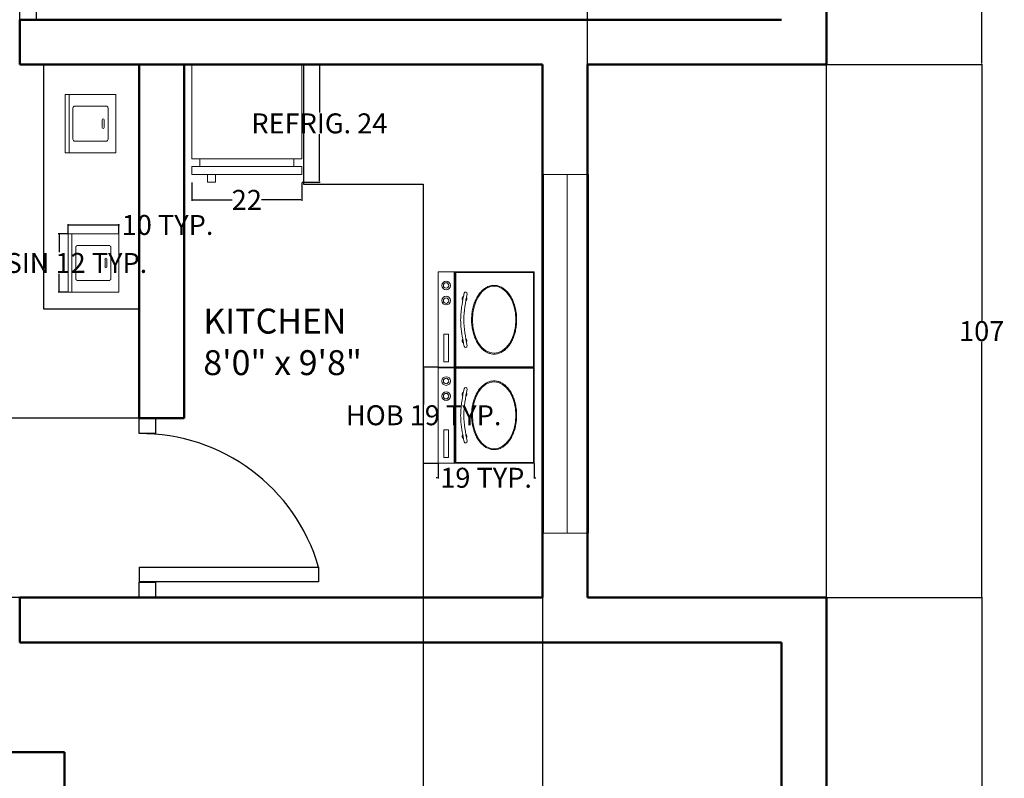
# Model space of a CAD drawing. Units: inches. Extents: x 870 to 1431, y 383 to 1070.
# Tile 8 of 9: x 1230 to 1428, y 604 to 756. Entities that reach past the tile are written whole.
import ezdxf

# ---------------------------------------------------------------- set-up
doc = ezdxf.new("R2010")
doc.units = ezdxf.units.IN
doc.header["$MEASUREMENT"] = 0
for name, color, linetype, lineweight in [('A-ANNO-DIMS', 2, 'Continuous', 18), ('A-AREA-IDEN', 7, 'Continuous', 25), ('A-DOOR', 3, 'Continuous', 25), ('A-EQPM', 8, 'Continuous', 20), ('A-FLOR-CASE', 9, 'Continuous', 25), ('A-FLOR-FIXT', 9, 'Continuous', 18), ('A-GLAZ', 4, 'Continuous', 18), ('A-WALL', 7, 'Continuous', 50)]:
    doc.layers.add(name, color=color, linetype=linetype, lineweight=lineweight)
doc.styles.get("Standard").update_dxf_attribs({"font": 'arial.ttf'})
doc.dimstyles.get("Standard").update_dxf_attribs({"dimtxt": 4, "dimasz": 0.18, "dimexe": 0.18, "dimexo": 0.0625, "dimgap": 0.09, "dimtad": 0, "dimtih": 1, "dimtoh": 1, "dimdec": 0, "dimrnd": 6, "dimzin": 0, "dimdsep": 46, "dimlunit": 3, "dimtxsty": 'Standard', "dimcen": 0.09, "dimadec": 0, "dimazin": 0, "dimtfac": 1, "dimtdec": 0, "dimtofl": 0, "dimtmove": 0, "dimatfit": 3, "dimfxl": 1, "dimtolj": 1, "dimtzin": 0, "dimarcsym": 0})

# ---------------------------------------------------------------- blocks, each defined once
blk = doc.blocks.new('A$C7E884C79')
for p, q in [((0, 0), (0, 600)), ((0, 600), (0, 0)), ((0, 600), (600, 600)), ((600, 600), (600, 0)), ((600, 0), (600, 600)), ((600, 600), (600, 450)), ((600, 600), (600, 500)), ((600, 500), (0, 500)), ((600, 495), (0, 495)), ((600, 500), (600, 0)), ((0, 0), (600, 0))]:
    blk.add_line(p, q)
for points in [[(36.4, 564.7), (208.9, 564.7), (208.9, 535.3), (36.4, 535.3)], [(5, 490), (595, 490), (595, 5), (5, 5)]]:
    blk.add_lwpolyline(points, close=True)
for centre, radius in [((419.3, 550), 27), ((419.3, 550), 17), ((513.9, 550), 27), ((513.9, 550), 17)]:
    blk.add_circle(centre, radius)
for centre, radius, start, end in [((137.2, 428), 10, 107.98291, 276.95811), ((168.5, 434.2), 15, 50.78881, 150.36701), ((431.5, 434.2), 15, 29.63299, 129.21119), ((462.8, 428), 10, 263.04189, 72.01709), ((168.5, 434.2), 15, 234.01645, 327.14121), ((431.5, 434.2), 15, 212.85879, 305.98355)]:
    blk.add_arc(centre, radius, start, end)
blk.add_ellipse((300, 250), major_axis=(-209.5, 0), ratio=0.648352)
for points, knots in [([(134.1, 437.5), (144.6, 439.5), (155.1, 441.6), (186, 447.3), (206.5, 450.9), (247.9, 456.4), (268.7, 458.3), (293.5, 458.9), (297.3, 458.9), (304.8, 458.9), (308.5, 458.8), (319.7, 458.5), (327.1, 458.1), (349.4, 456.5), (364.1, 454.9), (399.8, 449.9), (420.6, 446.2), (449.5, 440.7), (457.7, 439.1), (465.9, 437.5)], [0, 0, 0, 0, 31.638865, 31.638865, 92.600143, 92.600143, 153.561421, 153.561421, 164.367647, 164.367647, 175.173874, 175.173874, 196.786327, 196.786327, 240.011233, 240.011233, 302.099201, 302.099201, 326.773065, 326.773065, 326.773065, 326.773065]), ([(85.5, 250), (85.5, 244.8), (85.9, 239.6), (88, 226.9), (90.2, 219.4), (96.4, 204.8), (100.4, 197.7), (109.9, 184.1), (115.6, 177.5), (128.3, 165.1), (135.4, 159.2), (150.9, 148.3), (159.3, 143.3), (177.1, 134.2), (186.6, 130.1), (206.5, 123), (216.8, 119.9), (238.1, 114.9), (249, 113), (271.2, 110.2), (282.5, 109.4), (305, 109), (316.4, 109.4), (338.8, 111.3), (349.8, 112.8), (371.5, 117), (382.1, 119.6), (402.5, 126), (412.3, 129.7), (431, 138.1), (439.8, 142.8), (456.2, 153), (463.8, 158.6), (477.6, 170.5), (483.8, 176.8), (494.6, 190.1), (499.2, 197), (506.7, 211.3), (509.5, 218.7), (513.4, 233.6), (514.4, 241.3), (514.6, 256.5), (513.8, 264.1), (510.2, 279.1), (507.6, 286.6), (500.4, 300.9), (496, 307.9), (485.5, 321.3), (479.5, 327.7), (466, 339.7), (458.5, 345.3), (442.4, 355.8), (433.6, 360.5), (415.2, 369.1), (405.5, 373), (385.2, 379.5), (374.7, 382.3), (353.1, 386.7), (342, 388.3), (319.7, 390.5), (308.4, 390.9), (285.8, 390.7), (274.5, 390.1), (252.3, 387.5), (241.3, 385.7), (219.9, 380.9), (209.5, 378), (189.5, 371), (179.9, 367.1), (161.8, 358.1), (153.3, 353.2), (137.6, 342.5), (130.3, 336.7), (117.3, 324.4), (111.6, 317.9), (101.6, 304.3), (97.5, 297.3), (91, 282.8), (88.6, 275.3), (86, 261.9), (85.5, 255.9), (85.5, 250)], [0, 0, 0, 0, 0.108301, 0.108301, 0.267534, 0.267534, 0.426768, 0.426768, 0.586002, 0.586002, 0.745235, 0.745235, 0.904469, 0.904469, 1.063703, 1.063703, 1.222936, 1.222936, 1.38217, 1.38217, 1.541404, 1.541404, 1.700637, 1.700637, 1.859871, 1.859871, 2.019105, 2.019105, 2.178339, 2.178339, 2.337572, 2.337572, 2.496806, 2.496806, 2.65604, 2.65604, 2.815273, 2.815273, 2.974507, 2.974507, 3.133741, 3.133741, 3.292974, 3.292974, 3.452208, 3.452208, 3.611442, 3.611442, 3.770676, 3.770676, 3.929909, 3.929909, 4.089143, 4.089143, 4.248377, 4.248377, 4.40761, 4.40761, 4.566844, 4.566844, 4.726078, 4.726078, 4.885311, 4.885311, 5.044545, 5.044545, 5.203779, 5.203779, 5.363012, 5.363012, 5.522246, 5.522246, 5.68148, 5.68148, 5.840714, 5.840714, 5.999947, 5.999947, 6.159181, 6.159181, 6.283185, 6.283185, 6.283185, 6.283185])]:
    blk.add_open_spline(points, degree=3, knots=knots)
blk.add_open_spline([(138, 417.8), (192, 428.4), (300, 449.4), (408, 428.4), (462, 417.8)], degree=3)
blk = doc.blocks.new('REFRI-00')
for points in [[(-0.35, 0.35), (-0.35, -0.25), (0.35, -0.25), (0.35, 0.35), (-0.35, 0.35)], [(-0.3, -0.3), (-0.3, -0.25)], [(0.3, -0.3), (0.3, -0.25)], [(-0.35, -0.3), (-0.35, -0.35), (0.35, -0.35), (0.35, -0.3), (-0.35, -0.3)], [(-0.25, -0.35), (-0.25, -0.4), (-0.2, -0.4), (-0.2, -0.35)]]:
    blk.add_lwpolyline(points)
blk = doc.blocks.new('LAVAD-01')
for p, q in [((-0.322, 0.358), (-0.322, -0.392)), ((0.328, 0.358), (-0.322, 0.358)), ((-0.272, 0.358), (-0.272, -0.392)), ((0.328, -0.392), (0.328, 0.358)), ((-0.222, 0.183), (-0.222, -0.217)), ((0.203, 0.208), (-0.197, 0.208)), ((0.228, -0.217), (0.228, 0.183)), ((0.153, 0.033), (0.153, -0.067)), ((0.165, 0.046), (0.165, 0.046)), ((0.178, -0.067), (0.178, 0.033)), ((0.165, -0.079), (0.165, -0.079)), ((-0.197, -0.242), (0.203, -0.242)), ((-0.322, -0.392), (0.328, -0.392))]:
    blk.add_line(p, q)
for centre, radius, start, end in [((-0.197, 0.183), 0.025, 90, 180), ((0.203, 0.183), 0.025, 0, 90), ((0.165, 0.033), 0.0125, 90, 180), ((0.165, 0.033), 0.0125, 0, 90), ((0.165, -0.067), 0.0125, 180, 270), ((0.165, -0.067), 0.0125, 270, 360), ((-0.197, -0.217), 0.025, 180, 270), ((0.203, -0.217), 0.025, 270, 360)]:
    blk.add_arc(centre, radius, start, end)
blk = doc.blocks.new('WIN-72IN')
blk.add_line((4.72, 72), (4.72, 0))
blk.add_lwpolyline([(0, 72), (9, 72), (9, 0), (0, 0)], close=True)
blk = doc.blocks.new('*D109')
at = {"layer": 'A-ANNO-DIMS', "color": 0, "lineweight": -2, "transparency": 16777216}
for p, q in [((1313.73, 686.72), (1310.72, 686.72)), ((1310.9, 686.54), (1310.9, 679.24)), ((1310.9, 667.61), (1310.9, 674.92)), ((1313.73, 667.43), (1310.72, 667.43))]:
    blk.add_line(p, q, dxfattribs=at)
at = {"layer": 'A-ANNO-DIMS', "color": 0, "transparency": 16777216}
for points in [[(1310.87, 686.54), (1310.93, 686.54), (1310.9, 686.72)], [(1310.87, 667.61), (1310.93, 667.61), (1310.9, 667.43)]]:
    blk.add_solid(points, dxfattribs=at)
at = {"layer": 'Defpoints', "color": 0, "transparency": 16777216}
for p in [(1310.9, 686.72), (1313.8, 686.72), (1313.8, 667.43)]:
    blk.add_point(p, dxfattribs=at)
at = {"layer": 'A-ANNO-DIMS', "color": 0, "transparency": 16777216, "insert": (1310.9, 677.08), "char_height": 4, "attachment_point": 5}
blk.add_mtext('\\A1;HOB 19 TYP.', dxfattribs=at)
blk = doc.blocks.new('*D110')
at = {"layer": 'A-ANNO-DIMS', "color": 0, "lineweight": -2, "transparency": 16777216}
for p, q in [((1313.8, 667.37), (1313.8, 664.36)), ((1333.09, 667.37), (1333.09, 664.36)), ((1313.62, 664.54), (1313.44, 664.54)), ((1333.27, 664.54), (1333.45, 664.54))]:
    blk.add_line(p, q, dxfattribs=at)
at = {"layer": 'A-ANNO-DIMS', "color": 0, "transparency": 16777216}
for points in [[(1313.62, 664.57), (1313.62, 664.51), (1313.8, 664.54)], [(1333.27, 664.57), (1333.27, 664.51), (1333.09, 664.54)]]:
    blk.add_solid(points, dxfattribs=at)
at = {"layer": 'Defpoints', "color": 0, "transparency": 16777216}
for p in [(1313.8, 667.43), (1333.09, 667.43), (1313.8, 664.54)]:
    blk.add_point(p, dxfattribs=at)
at = {"layer": 'A-ANNO-DIMS', "color": 0, "transparency": 16777216, "insert": (1323.44, 664.54), "char_height": 4, "attachment_point": 5}
blk.add_mtext('\\A1;19 TYP.', dxfattribs=at)
blk = doc.blocks.new('*D117')
at = {"layer": 'A-ANNO-DIMS', "color": 0, "lineweight": -2, "transparency": 16777216}
for p, q in [((1239.42, 713.52), (1237.54, 713.52)), ((1237.72, 713.34), (1237.72, 709.81)), ((1237.72, 701.96), (1237.72, 705.49)), ((1239.42, 701.78), (1237.54, 701.78))]:
    blk.add_line(p, q, dxfattribs=at)
at = {"layer": 'A-ANNO-DIMS', "color": 0, "transparency": 16777216}
for points in [[(1237.69, 713.34), (1237.75, 713.34), (1237.72, 713.52)], [(1237.69, 701.96), (1237.75, 701.96), (1237.72, 701.78)]]:
    blk.add_solid(points, dxfattribs=at)
at = {"layer": 'Defpoints', "color": 0, "transparency": 16777216}
for p in [(1237.72, 713.52), (1239.49, 713.52), (1239.49, 701.78)]:
    blk.add_point(p, dxfattribs=at)
at = {"layer": 'A-ANNO-DIMS', "color": 0, "transparency": 16777216, "insert": (1237.72, 707.65), "char_height": 4, "attachment_point": 5}
blk.add_mtext('\\A1;BASIN 12 TYP.', dxfattribs=at)
blk = doc.blocks.new('*D118')
at = {"layer": 'A-ANNO-DIMS', "color": 0, "lineweight": -2, "transparency": 16777216}
for p, q in [((1239.49, 713.58), (1239.49, 715.46)), ((1239.67, 715.28), (1249.48, 715.28)), ((1249.66, 713.58), (1249.66, 715.46)), ((1249.66, 715.28), (1249.84, 715.28))]:
    blk.add_line(p, q, dxfattribs=at)
at = {"layer": 'A-ANNO-DIMS', "color": 0, "transparency": 16777216}
for points in [[(1239.67, 715.31), (1239.67, 715.25), (1239.49, 715.28)], [(1249.48, 715.31), (1249.48, 715.25), (1249.66, 715.28)]]:
    blk.add_solid(points, dxfattribs=at)
at = {"layer": 'Defpoints', "color": 0, "transparency": 16777216}
for p in [(1249.66, 715.28), (1239.49, 713.52), (1249.66, 713.52)]:
    blk.add_point(p, dxfattribs=at)
at = {"layer": 'A-ANNO-DIMS', "color": 0, "transparency": 16777216, "insert": (1259.48, 715.28), "char_height": 4, "attachment_point": 5}
blk.add_mtext('\\A1;10 TYP.', dxfattribs=at)
blk = doc.blocks.new('*D121')
at = {"layer": 'A-ANNO-DIMS', "color": 0, "lineweight": -2, "transparency": 16777216}
for p, q in [((1286.48, 747.48), (1290.14, 747.48)), ((1289.96, 747.3), (1289.96, 737.82)), ((1289.96, 724.04), (1289.96, 733.51)), ((1286.48, 723.86), (1290.14, 723.86))]:
    blk.add_line(p, q, dxfattribs=at)
at = {"layer": 'A-ANNO-DIMS', "color": 0, "transparency": 16777216}
for points in [[(1289.93, 747.3), (1289.99, 747.3), (1289.96, 747.48)], [(1289.93, 724.04), (1289.99, 724.04), (1289.96, 723.86)]]:
    blk.add_solid(points, dxfattribs=at)
at = {"layer": 'Defpoints', "color": 0, "transparency": 16777216}
for p in [(1286.42, 747.48), (1289.96, 747.48), (1286.42, 723.86)]:
    blk.add_point(p, dxfattribs=at)
at = {"layer": 'A-ANNO-DIMS', "color": 0, "transparency": 16777216, "insert": (1289.96, 735.67), "char_height": 4, "attachment_point": 5}
blk.add_mtext('\\A1;REFRIG. 24', dxfattribs=at)
blk = doc.blocks.new('*D122')
at = {"layer": 'A-ANNO-DIMS', "color": 0, "lineweight": -2, "transparency": 16777216}
for p, q in [((1264.37, 723.79), (1264.37, 720.13)), ((1286.42, 723.79), (1286.42, 720.13)), ((1264.55, 720.31), (1272.43, 720.31)), ((1286.24, 720.31), (1278.36, 720.31))]:
    blk.add_line(p, q, dxfattribs=at)
at = {"layer": 'A-ANNO-DIMS', "color": 0, "transparency": 16777216}
for points in [[(1264.55, 720.34), (1264.55, 720.28), (1264.37, 720.31)], [(1286.24, 720.34), (1286.24, 720.28), (1286.42, 720.31)]]:
    blk.add_solid(points, dxfattribs=at)
at = {"layer": 'Defpoints', "color": 0, "transparency": 16777216}
for p in [(1264.37, 723.86), (1286.42, 723.86), (1286.42, 720.31)]:
    blk.add_point(p, dxfattribs=at)
at = {"layer": 'A-ANNO-DIMS', "color": 0, "transparency": 16777216, "insert": (1275.39, 720.31), "char_height": 4, "attachment_point": 5}
blk.add_mtext('\\A1;22', dxfattribs=at)
blk = doc.blocks.new('*D133')
at = {"layer": 'A-ANNO-DIMS', "color": 0, "lineweight": -2, "transparency": 16777216}
for p, q in [((1382.85, 916.48), (1423.14, 916.48)), ((1422.96, 916.3), (1422.96, 834.11)), ((1422.96, 747.66), (1422.96, 829.84)), ((1391.85, 747.48), (1423.14, 747.48))]:
    blk.add_line(p, q, dxfattribs=at)
at = {"layer": 'A-ANNO-DIMS', "color": 0, "transparency": 16777216}
for points in [[(1422.93, 916.3), (1422.99, 916.3), (1422.96, 916.48)], [(1422.93, 747.66), (1422.99, 747.66), (1422.96, 747.48)]]:
    blk.add_solid(points, dxfattribs=at)
at = {"layer": 'Defpoints', "color": 0, "transparency": 16777216}
for p in [(1382.79, 916.48), (1391.79, 747.48), (1422.96, 747.48)]:
    blk.add_point(p, dxfattribs=at)
at = {"layer": 'A-ANNO-DIMS', "color": 0, "transparency": 16777216, "insert": (1422.96, 831.98), "char_height": 4, "attachment_point": 5}
blk.add_mtext('\\A1;169', dxfattribs=at)
blk = doc.blocks.new('*D134')
at = {"layer": 'A-ANNO-DIMS', "color": 0, "lineweight": -2, "transparency": 16777216}
for p, q in [((1391.85, 640.48), (1423.14, 640.48)), ((1422.96, 640.3), (1422.96, 554.08)), ((1422.96, 463.66), (1422.96, 549.88)), ((1391.85, 463.48), (1423.14, 463.48))]:
    blk.add_line(p, q, dxfattribs=at)
at = {"layer": 'A-ANNO-DIMS', "color": 0, "transparency": 16777216}
for points in [[(1422.93, 640.3), (1422.99, 640.3), (1422.96, 640.48)], [(1422.93, 463.66), (1422.99, 463.66), (1422.96, 463.48)]]:
    blk.add_solid(points, dxfattribs=at)
at = {"layer": 'Defpoints', "color": 0, "transparency": 16777216}
for p in [(1391.79, 640.48), (1391.79, 463.48), (1422.96, 463.48)]:
    blk.add_point(p, dxfattribs=at)
at = {"layer": 'A-ANNO-DIMS', "color": 0, "transparency": 16777216, "insert": (1422.96, 551.98), "char_height": 4, "attachment_point": 5}
blk.add_mtext('\\A1;177', dxfattribs=at)
blk = doc.blocks.new('*D138')
at = {"layer": 'A-ANNO-DIMS', "color": 0, "lineweight": -2, "transparency": 16777216}
for p, q in [((1343.79, 640.54), (1343.79, 1067.52)), ((1343.97, 1067.34), (1364.75, 1067.34)), ((1391.61, 1067.34), (1370.83, 1067.34)), ((1391.79, 640.54), (1391.79, 1067.52))]:
    blk.add_line(p, q, dxfattribs=at)
at = {"layer": 'A-ANNO-DIMS', "color": 0, "transparency": 16777216}
for points in [[(1343.97, 1067.37), (1343.97, 1067.31), (1343.79, 1067.34)], [(1391.61, 1067.37), (1391.61, 1067.31), (1391.79, 1067.34)]]:
    blk.add_solid(points, dxfattribs=at)
at = {"layer": 'Defpoints', "color": 0, "transparency": 16777216}
for p in [(1391.79, 1067.34), (1343.79, 640.48), (1391.79, 640.48)]:
    blk.add_point(p, dxfattribs=at)
at = {"layer": 'A-ANNO-DIMS', "color": 0, "transparency": 16777216, "insert": (1367.79, 1067.34), "char_height": 4, "attachment_point": 5}
blk.add_mtext('\\A1;48', dxfattribs=at)
blk = doc.blocks.new('*D139')
at = {"layer": 'A-ANNO-DIMS', "color": 0, "lineweight": -2, "transparency": 16777216}
for p, q in [((1343.85, 747.48), (1423.14, 747.48)), ((1422.96, 747.3), (1422.96, 696.11)), ((1422.96, 640.66), (1422.96, 691.84)), ((1343.85, 640.48), (1423.14, 640.48))]:
    blk.add_line(p, q, dxfattribs=at)
at = {"layer": 'A-ANNO-DIMS', "color": 0, "transparency": 16777216}
for points in [[(1422.93, 747.3), (1422.99, 747.3), (1422.96, 747.48)], [(1422.93, 640.66), (1422.99, 640.66), (1422.96, 640.48)]]:
    blk.add_solid(points, dxfattribs=at)
at = {"layer": 'Defpoints', "color": 0, "transparency": 16777216}
for p in [(1343.79, 747.48), (1422.96, 747.48), (1343.79, 640.48)]:
    blk.add_point(p, dxfattribs=at)
at = {"layer": 'A-ANNO-DIMS', "color": 0, "transparency": 16777216, "insert": (1422.96, 693.98), "char_height": 4, "attachment_point": 5}
blk.add_mtext('\\A1;107', dxfattribs=at)
blk = doc.blocks.new('*D140')
at = {"layer": 'A-ANNO-DIMS', "color": 0, "lineweight": -2, "transparency": 16777216}
for p, q in [((1253.73, 676.48), (876.24, 676.48)), ((876.42, 676.3), (876.42, 660.61)), ((876.42, 640.66), (876.42, 656.34)), ((1253.73, 640.48), (876.24, 640.48))]:
    blk.add_line(p, q, dxfattribs=at)
at = {"layer": 'A-ANNO-DIMS', "color": 0, "transparency": 16777216}
for points in [[(876.39, 676.3), (876.45, 676.3), (876.42, 676.48)], [(876.39, 640.66), (876.45, 640.66), (876.42, 640.48)]]:
    blk.add_solid(points, dxfattribs=at)
at = {"layer": 'Defpoints', "color": 0, "transparency": 16777216}
for p in [(876.42, 676.48), (1253.79, 676.48), (1253.79, 640.48)]:
    blk.add_point(p, dxfattribs=at)
at = {"layer": 'A-ANNO-DIMS', "color": 0, "transparency": 16777216, "insert": (876.42, 658.48), "char_height": 4, "attachment_point": 5}
blk.add_mtext('\\A1;36', dxfattribs=at)
blk = doc.blocks.new('*D141')
at = {"layer": 'A-ANNO-DIMS', "color": 0, "lineweight": -2, "transparency": 16777216}
for p, q in [((1310.79, 640.41), (1310.79, 385.26)), ((1334.79, 640.41), (1334.79, 385.26)), ((1310.97, 385.44), (1319.81, 385.44)), ((1334.61, 385.44), (1325.77, 385.44))]:
    blk.add_line(p, q, dxfattribs=at)
at = {"layer": 'A-ANNO-DIMS', "color": 0, "transparency": 16777216}
for points in [[(1310.97, 385.47), (1310.97, 385.41), (1310.79, 385.44)], [(1334.61, 385.47), (1334.61, 385.41), (1334.79, 385.44)]]:
    blk.add_solid(points, dxfattribs=at)
at = {"layer": 'Defpoints', "color": 0, "transparency": 16777216}
for p in [(1310.79, 640.48), (1334.79, 640.48), (1334.79, 385.44)]:
    blk.add_point(p, dxfattribs=at)
at = {"layer": 'A-ANNO-DIMS', "color": 0, "transparency": 16777216, "insert": (1322.79, 385.44), "char_height": 4, "attachment_point": 5}
blk.add_mtext('\\A1;24', dxfattribs=at)

msp = doc.modelspace()

# ---------------------------------------------------------------- linework, layer by layer
at = {"layer": 'A-DOOR'}
for points in [[(1233.0601, 756.4772), (1229.7907, 756.4772), (1229.7907, 759.5786), (1233.0601, 759.5786)], [(1257.0319, 673.3878), (1253.7626, 673.3878), (1253.7626, 676.4891), (1257.0319, 676.4891)], [(1253.8163, 646.6227), (1289.8163, 646.6227), (1289.8163, 643.6227), (1253.8163, 643.6227)], [(1257.0601, 640.4772), (1253.7907, 640.4772), (1253.7907, 643.5786), (1257.0601, 643.5786)]]:
    msp.add_lwpolyline(points, close=True, dxfattribs=at)
msp.add_arc((1254.126, 636.2118), 37.1777, 16.261985, 90.560099, dxfattribs=at)
at = {"layer": 'A-FLOR-CASE'}
for p, q in [((1234.5907, 747.4772), (1234.5907, 698.4402)), ((1286.7907, 747.4772), (1286.7907, 723.4772)), ((1286.7907, 723.4772), (1310.7907, 723.4772)), ((1310.7907, 723.4772), (1310.7907, 640.4772)), ((1234.5907, 698.4402), (1253.7907, 698.4402))]:
    msp.add_line(p, q, dxfattribs=at)
at = {"layer": 'A-WALL'}
for p, q in [((1391.7907, 952.4772), (1391.7907, 747.4772)), ((1229.7907, 756.4772), (1382.7907, 756.4772)), ((1229.7907, 756.4772), (1229.7907, 747.4772)), ((1229.7907, 756.4772), (1229.7907, 747.4772)), ((1229.7907, 747.4772), (1334.7907, 747.4772)), ((1253.7907, 747.4772), (1253.7907, 676.4772)), ((1262.7907, 747.4772), (1262.7907, 676.4772)), ((1334.7907, 747.4772), (1334.7907, 640.4772)), ((1343.7907, 747.4772), (1343.7907, 640.4772)), ((1343.7907, 747.4772), (1391.7907, 747.4772)), ((1253.7907, 676.4772), (1262.7907, 676.4772)), ((1229.7907, 640.4772), (1229.7907, 631.4772)), ((1229.7907, 640.4772), (1229.7907, 631.4772)), ((1229.7907, 640.4772), (1253.7907, 640.4772)), ((1253.7907, 640.4772), (1334.7907, 640.4772)), ((1343.7907, 640.4772), (1391.7907, 640.4772)), ((1391.7907, 640.4772), (1391.7907, 463.4772)), ((1229.7907, 631.4772), (1334.7907, 631.4772)), ((1334.7907, 631.4772), (1382.7907, 631.4772)), ((1382.7907, 631.4772), (1382.7907, 472.4772)), ((1193.7907, 609.4772), (1238.7907, 609.4772)), ((1238.7907, 609.4772), (1238.7907, 463.4772))]:
    msp.add_line(p, q, dxfattribs=at)

# ---------------------------------------------------------------- block references
at = {"layer": 'A-EQPM', "xscale": 31.49606299212599, "yscale": 31.49606299212599, "zscale": 31.49606299212599}
msp.add_blockref('REFRI-00', (1275.3947, 736.4536), dxfattribs=at)
at = {"layer": 'A-EQPM', "xscale": 0.0321522309711237, "yscale": 0.0321522309711237, "zscale": 0.0321522309711237, "rotation": 90}
for p in [(1333.0878, 686.6097), (1333.0878, 686.6097), (1333.0878, 667.4328), (1333.0878, 667.4328)]:
    msp.add_blockref('A$C7E884C79', p, dxfattribs=at)
at = {"layer": 'A-FLOR-FIXT', "xscale": 15.65193150862309, "yscale": 15.65193150862309, "zscale": 15.65193150862309}
for p in [(1243.9574, 735.8806), (1244.5263, 707.908)]:
    msp.add_blockref('LAVAD-01', p, dxfattribs=at)
at = {"layer": 'A-GLAZ'}
msp.add_blockref('WIN-72IN', (1334.973, 653.414), dxfattribs=at)

# ---------------------------------------------------------------- texts
at = {"layer": 'A-AREA-IDEN', "insert": (1266.6555, 698.4768), "char_height": 5, "attachment_point": 1}
msp.add_mtext_dynamic_manual_height_columns('KITCHEN\\P8\'0" x 9\'8"', width=69.132678, gutter_width=1, heights=[0], dxfattribs=at)

# ---------------------------------------------------------------- dimensions: what is measured, and where the dimension line sits
at = {"layer": 'A-ANNO-DIMS'}
for base, p1, p2, picture, middle in [((1391.7907, 1067.3407), (1343.7907, 640.4772), (1391.7907, 640.4772), '*D138', (1367.7907, 1067.3407)), ((1286.4183, 720.3119), (1264.3711, 723.8552), (1286.4183, 723.8552), '*D122', (1275.3947, 720.3119)), ((1334.7907, 385.44), (1310.7907, 640.4772), (1334.7907, 640.4772), '*D141', (1322.7907, 385.44))]:
    dim = msp.add_linear_dim(base=base, p1=p1, p2=p2, dimstyle='Standard', override={"dimdec": 0, "dimlfac": 1, "dimrnd": 0, "dimzin": 0, "dimdsep": 46, "dimlunit": 2}, dxfattribs=at)
    dim.commit()
    dim.dimension.update_dxf_attribs({"geometry": picture, "text_midpoint": middle})
for base, p1, p2, picture, middle in [((1422.9581, 747.4772), (1382.7907, 916.4772), (1391.7907, 747.4772), '*D133', (1422.9581, 831.9772)), ((1422.9581, 747.4772), (1343.7907, 640.4772), (1343.7907, 747.4772), '*D139', (1422.9581, 693.9772)), ((876.4215, 676.4772), (1253.7907, 640.4772), (1253.7907, 676.4772), '*D140', (876.4215, 658.4772)), ((1422.9581, 463.4772), (1391.7907, 640.4772), (1391.7907, 463.4772), '*D134', (1422.9581, 551.9772))]:
    dim = msp.add_linear_dim(base=base, p1=p1, p2=p2, angle=90, dimstyle='Standard', override={"dimdec": 0, "dimlfac": 1, "dimrnd": 0, "dimzin": 0, "dimdsep": 46, "dimlunit": 2}, dxfattribs=at)
    dim.commit()
    dim.dimension.update_dxf_attribs({"geometry": picture, "text_midpoint": middle})
for base, p1, p2, angle, text, picture, middle in [((1289.9616, 747.4772), (1286.4183, 723.8552), (1286.4183, 747.4772), 90, 'REFRIG. <>', '*D121', (1289.9616, 735.6662)), ((1237.7245, 713.5187), (1239.4853, 701.7797), (1239.4853, 713.5187), 90, 'BASIN <> TYP.', '*D117', (1237.7245, 707.6492)), ((1310.9027, 686.7241), (1313.7964, 667.4328), (1313.7964, 686.7241), 90, 'HOB <> TYP.', '*D109', (1310.9027, 677.0784)), ((1313.7964, 664.5391), (1333.0878, 667.4328), (1313.7964, 667.4328), 180, '<> TYP.', '*D110', (1323.4421, 664.5391))]:
    dim = msp.add_linear_dim(base=base, p1=p1, p2=p2, angle=angle, text=text, dimstyle='Standard', override={"dimdec": 0, "dimlfac": 1, "dimrnd": 0, "dimzin": 0, "dimdsep": 46, "dimlunit": 2}, dxfattribs=at)
    dim.commit()
    dim.dimension.update_dxf_attribs({"geometry": picture, "text_midpoint": middle})
dim = msp.add_linear_dim(base=(1249.6591, 715.2795), p1=(1239.4853, 713.5187), p2=(1249.6591, 713.5187), text='<> TYP.', dimstyle='Standard', override={"dimdec": 0, "dimlfac": 1, "dimrnd": 0, "dimzin": 0, "dimdsep": 46, "dimlunit": 2}, dxfattribs=at)
dim.commit()
dim.dimension.update_dxf_attribs({"geometry": '*D118', "text_midpoint": (1259.4762, 715.2795)})

doc.saveas('drawing.dxf')
